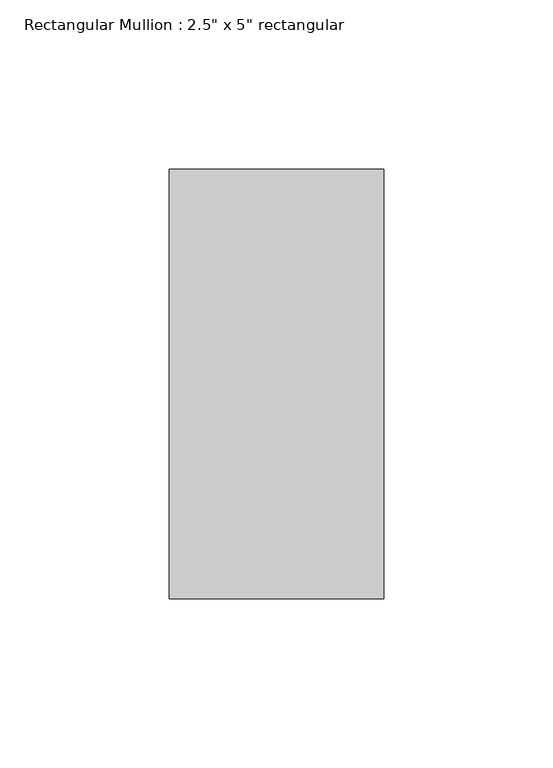
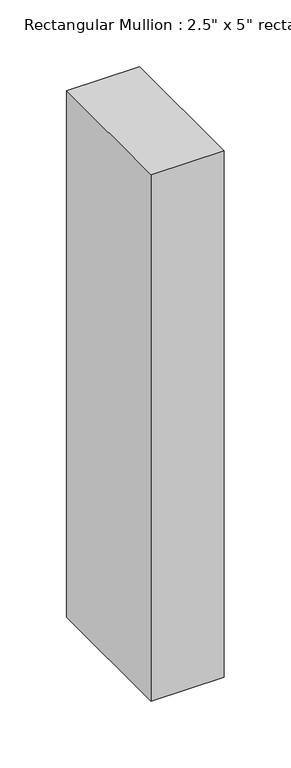
"""IFC4 building model written with IfcOpenShell, lengths in millimetres: member geometry."""

from ifc_helpers import new_model, si_unit, frame, origin, place, context, project, spatial, polyline, outline, extrude, source, transform, mapped, element, save


def member_86d06fe4(model_context):
    return source(origin(), model_context, "Body", "SweptSolid", [
        extrude(outline(polyline([(0.0, 63.5), (0.0, -63.5), (-63.5, -63.5), (-63.5, 63.5), (0.0, 63.5)])), frame((0.0, 0.0, -482.6), z_axis=(0.0, 0.0, 1.0), x_axis=(1.0, 0.0, 0.0)), (0.0, 0.0, 1.0), 482.6),
    ])


if __name__ == "__main__":
    model = new_model("IFC4")
    model_context = context("Model", 3, world=origin())
    ifc_project = project(units=[si_unit("LENGTHUNIT", "METRE", prefix="MILLI")], contexts=[model_context])
    site = spatial("IfcSite", under=ifc_project)
    building = spatial("IfcBuilding", under=site)
    placement = place(None, origin())
    member_shape = member_86d06fe4(model_context)
    element("IfcMember", 1, ObjectType="Rectangular Mullion : 2.5\" x 5\" rectangular", at=placement, inside=building, context=model_context, shape_type="MappedRepresentation", body=[
        mapped(member_shape, transform((0.0, 0.0, 0.0), x_axis=(1.0, 0.0, 0.0), y_axis=(0.0, 1.0, 0.0), z_axis=(0.0, 0.0, 1.0))),
    ])
    save(model, "model.ifc")

# Revit data of these elements
# Type "Rectangular Mullion : 2.5\" x 5\" rectangular"
#   built-in parameter 1007304 = 0.416667 (stored number, unit not read)
#   built-in parameter 1007301 = 0.104167 (stored number, unit not read)
#   built-in parameter 1007300 = 0.104167 (stored number, unit not read)
# Element 1 (IfcMember, "Rectangular Mullion : 2.5\" x 5\" rectangular")
#   Materials on its faces: "Door - Frame"
# Materials
#   "Door - Frame": colour RGB 118 70 51, transparency 0, Cost = 0
